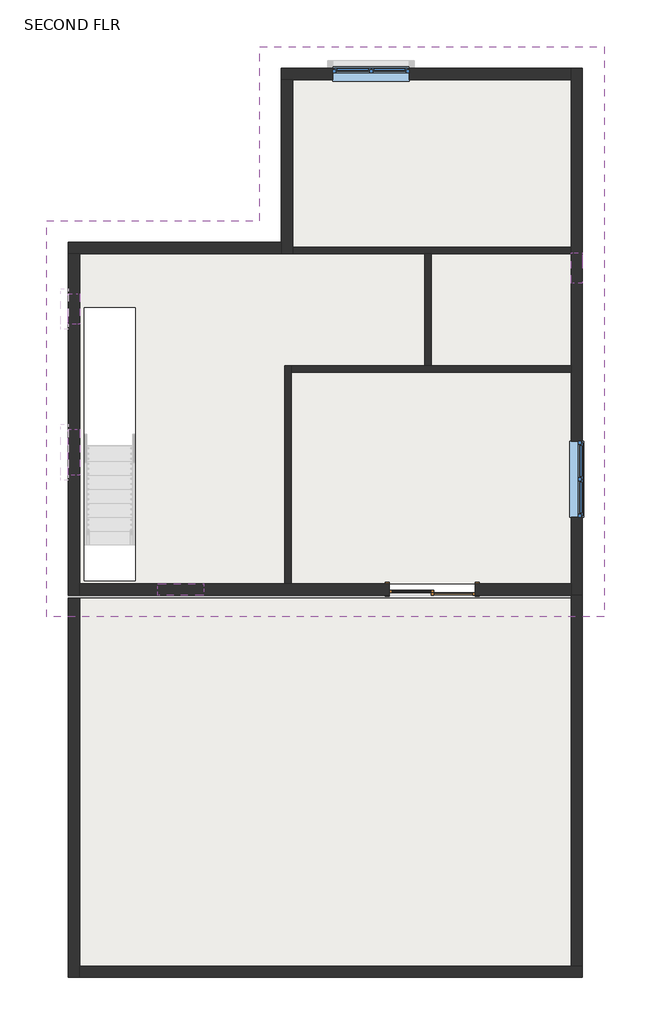
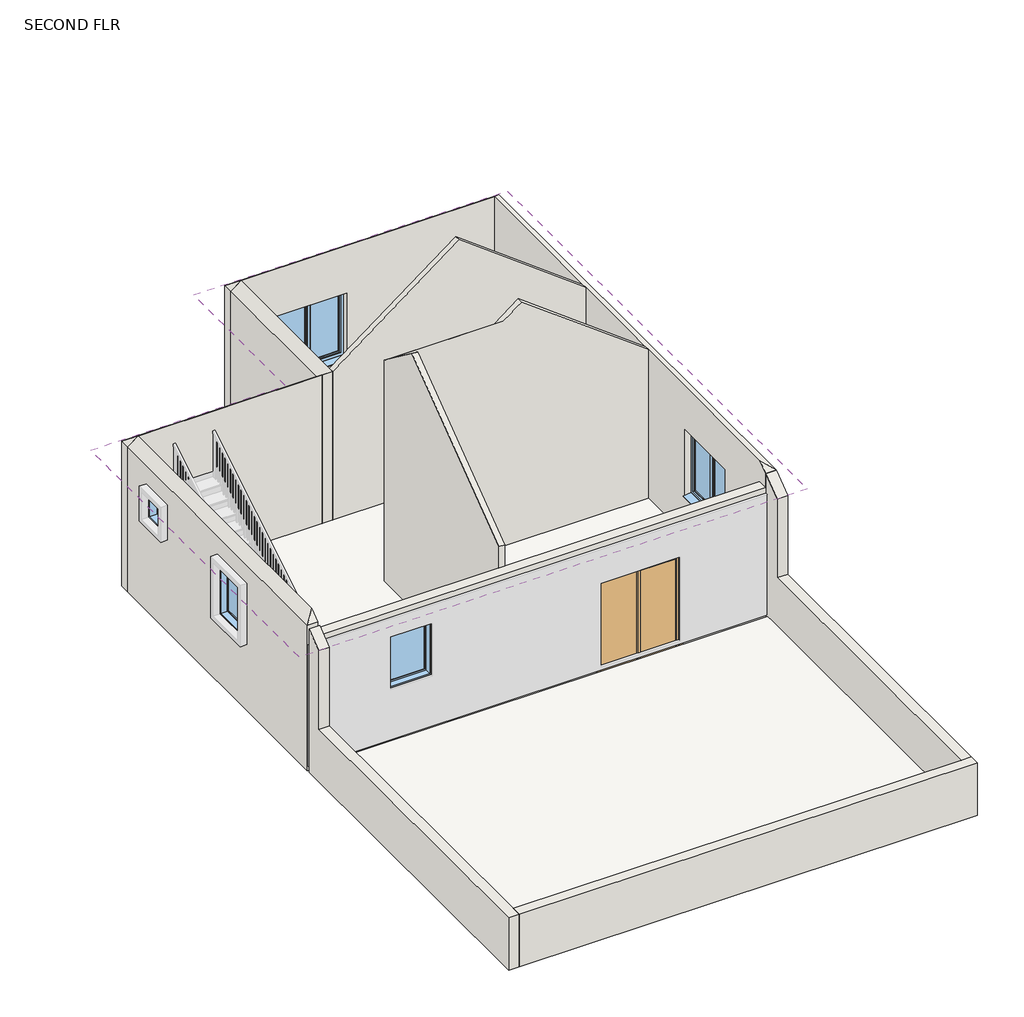
# One storey, part 1 of 2: 13 walls, 6 windows, 1 door, 1 roof, 1 slab.
"""IFC4 building model written with IfcOpenShell, lengths in millimetres."""

from ifc_helpers import new_model, si_unit, frame, origin, place, context, project, spatial, polyline, outline, extrude, faceted_brep, transform, mapped, element, save
from components import door_45189e27, window_80340324, fixed_window_3_x_3_dcb239d8, w2_windows_5_x_5_8ac21896

model = new_model("IFC4")

# Units and contexts
model_context = context("Model", 3, world=origin())
ifc_project = project(units=[si_unit("LENGTHUNIT", "METRE", prefix="MILLI")], contexts=[model_context])

# Site, building, storey
site = spatial("IfcSite", under=ifc_project)
building = spatial("IfcBuilding", under=site)
storey = spatial("IfcBuildingStorey", under=building, Name="SECOND FLR", Elevation=6400.8)

# Door
placement = place(None, origin())
door_shape = door_45189e27(model_context)
element("IfcDoor", 1, ObjectType="Door-Double-Sliding : 68\" x 84\"", at=placement, inside=storey, context=model_context, shape_type="MappedRepresentation", body=[
    mapped(door_shape, transform((1186.0219693, 1968.5641252, 6400.8), x_axis=(-1.0, 0.0, 0.0), y_axis=(0.0, -1.0, 0.0), z_axis=(0.0, 0.0, 1.0))),
])

# Roof
element("IfcRoof", 2, ObjectType="ROOFING 1'", at=placement, inside=storey, context=model_context, shape_type="Brep", body=[
    faceted_brep([(-2262.0280307, 9220.2641252, 9448.8), (-2262.0280307, 12700.0641252, 9448.8), (1179.6719693, 9258.3641252, 12030.075), (1179.6719693, 5778.5641252, 12030.075), (658.9719693, 5257.8641252, 12420.6), (-2566.8280307, 5257.8641252, 12420.6), (-6529.2280307, 9220.2641252, 9448.8), (4621.3719693, 12700.0641252, 9448.8), (-6529.2280307, 1295.4641252, 9448.8), (4621.3719693, 1295.4641252, 9448.8), (-2262.0280307, 9220.2641252, 9829.8), (1179.6719693, 5778.5641252, 12411.075), (1179.6719693, 9258.3641252, 12411.075), (-2262.0280307, 12700.0641252, 9829.8), (-6529.2280307, 9220.2641252, 9829.8), (-2566.8280307, 5257.8641252, 12801.6), (658.9719693, 5257.8641252, 12801.6), (4621.3719693, 12700.0641252, 9829.8), (-6529.2280307, 1295.4641252, 9829.8), (4621.3719693, 1295.4641252, 9829.8)], [[[0, 1, 2, 3]], [[0, 3, 4, 5, 6]], [[7, 2, 1]], [[8, 5, 4, 9]], [[6, 5, 8]], [[9, 4, 3, 2, 7]], [[10, 11, 12, 13]], [[10, 14, 15, 16, 11]], [[17, 13, 12]], [[18, 19, 16, 15]], [[14, 18, 15]], [[19, 17, 12, 11, 16]], [[6, 14, 10, 0]], [[8, 18, 14, 6]], [[9, 19, 18, 8]], [[7, 17, 19, 9]], [[1, 13, 17, 7]], [[0, 10, 13, 1]]]),
])

# Slab
element("IfcSlab", 3, ObjectType="MARBLE 6\"", at=placement, inside=storey, context=model_context, shape_type="SweptSolid", body=[
    extrude(outline(polyline([(3960.9719693, 12039.6641252), (3960.9719693, 8686.8641252), (-1601.6280307, 8686.8641252), (-1601.6280307, 12039.6641252), (3960.9719693, 12039.6641252)])), frame((0.0, 0.0, 6350.0), z_axis=(0.0, 0.0, 1.0), x_axis=(1.0, 0.0, 0.0)), (0.0, 0.0, 1.0), 152.4),
    extrude(outline(polyline([(3960.9719693, 8559.8641252), (3960.9719693, 6311.9641252), (1166.9719693, 6311.9641252), (1166.9719693, 8559.8641252), (3960.9719693, 8559.8641252)])), frame((0.0, 0.0, 6350.0), z_axis=(0.0, 0.0, 1.0), x_axis=(1.0, 0.0, 0.0)), (0.0, 0.0, 1.0), 152.4),
    extrude(outline(polyline([(3960.9719693, 1955.8641252), (-1639.7280307, 1955.8641252), (-1639.7280307, 6184.9641252), (3960.9719693, 6184.9641252), (3960.9719693, 1955.8641252)])), frame((0.0, 0.0, 6350.0), z_axis=(0.0, 0.0, 1.0), x_axis=(1.0, 0.0, 0.0)), (0.0, 0.0, 1.0), 152.4),
    extrude(outline(polyline([(1039.9719693, 8559.8641252), (1039.9719693, 6311.9641252), (-1766.7280307, 6311.9641252), (-1766.7280307, 1955.8641252), (-5868.7932997, 1955.8641252), (-5868.7932997, 8559.8641252), (1039.9719693, 8559.8641252)]), holes=[polyline([(-4756.3875748, 7481.7325341), (-5772.3875748, 7481.7325341), (-5772.3875748, 2020.7325341), (-4756.3875748, 2020.7325341), (-4756.3875748, 7481.7325341)])]), frame((0.0, 0.0, 6350.0), z_axis=(0.0, 0.0, 1.0), x_axis=(1.0, 0.0, 0.0)), (0.0, 0.0, 1.0), 152.4),
    extrude(outline(polyline([(-5868.7932997, 1663.7641252), (3960.9719693, 1663.7641252), (3960.9719693, -5689.5358748), (-5868.7932997, -5689.5358748), (-5868.7932997, 1663.7641252)])), frame((0.0, 0.0, 6350.0), z_axis=(0.0, 0.0, 1.0), x_axis=(1.0, 0.0, 0.0)), (0.0, 0.0, 1.0), 152.4),
])

# Walls
element("IfcWall", 4, ObjectType="INNER WALL5\"", at=placement, inside=storey, context=model_context, shape_type="Brep", body=[
    faceted_brep([(-1601.6280307, 8559.8641252, 6400.8), (1039.9719693, 8559.8641252, 6400.8), (1166.9719693, 8559.8641252, 6400.8), (3960.9719693, 8559.8641252, 6400.8), (3960.9719693, 8559.8641252, 9944.1), (1179.6719693, 8559.8641252, 12030.075), (-1601.6280307, 8559.8641252, 9944.1), (-1601.6280307, 8686.8641252, 6400.8), (-1601.6280307, 8686.8641252, 9944.1), (1179.6719693, 8686.8641252, 12030.075), (3960.9719693, 8686.8641252, 9944.1), (3960.9719693, 8686.8641252, 6400.8)], [[[0, 1, 2, 3, 4, 5, 6]], [[7, 8, 9, 10, 11]], [[3, 2, 1, 0, 7, 11]], [[4, 3, 11, 10]], [[0, 6, 8, 7]], [[6, 5, 9, 8]], [[5, 4, 10, 9]]]),
])
element("IfcWall", 5, ObjectType="INNER WALL5\"", at=placement, inside=storey, context=model_context, shape_type="Brep", body=[
    faceted_brep([(-1766.7280307, 6311.9641252, 6400.8), (-1766.7280307, 1955.8641252, 6400.8), (-1766.7280307, 1955.8641252, 9944.1), (-1766.7280307, 5257.8641252, 12420.6), (-1766.7280307, 6311.9641252, 11630.025), (-1639.7280307, 6311.9641252, 6400.8), (-1639.7280307, 6311.9641252, 11630.025), (-1639.7280307, 6184.9641252, 11725.275), (-1639.7280307, 5257.8641252, 12420.6), (-1639.7280307, 1955.8641252, 9944.1), (-1639.7280307, 1955.8641252, 6400.8), (-1639.7280307, 6184.9641252, 6400.8)], [[[0, 1, 2, 3, 4]], [[5, 6, 7, 8, 9, 10, 11]], [[1, 0, 5, 11, 10]], [[2, 1, 10, 9]], [[4, 3, 8, 7, 6]], [[3, 2, 9, 8]], [[0, 4, 6, 5]]]),
])
element("IfcWall", 6, ObjectType="INNER WALL5\"", at=placement, inside=storey, context=model_context, shape_type="Brep", body=[
    faceted_brep([(-1639.7280307, 6184.9641252, 6400.8), (3960.9719693, 6184.9641252, 6400.8), (3960.9719693, 6184.9641252, 9944.1), (1179.6719693, 6184.9641252, 12030.075), (773.2719693, 6184.9641252, 11725.275), (-1639.7280307, 6184.9641252, 11725.275), (-1639.7280307, 6311.9641252, 6400.8), (-1639.7280307, 6311.9641252, 11630.025), (646.2719693, 6311.9641252, 11630.025), (1179.6719693, 6311.9641252, 12030.075), (3960.9719693, 6311.9641252, 9944.1), (3960.9719693, 6311.9641252, 6400.8), (1166.9719693, 6311.9641252, 6400.8), (1039.9719693, 6311.9641252, 6400.8)], [[[0, 1, 2, 3, 4, 5]], [[6, 7, 8, 9, 10, 11, 12, 13]], [[1, 0, 6, 13, 12, 11]], [[2, 1, 11, 10]], [[5, 4, 8, 7]], [[4, 3, 9, 8]], [[3, 2, 10, 9]], [[0, 5, 7, 6]]]),
])
element("IfcWall", 7, ObjectType="INNER WALL5\"", at=placement, inside=storey, context=model_context, shape_type="SweptSolid", body=[
    extrude(outline(polyline([(1039.9719693, 6311.9641252), (1039.9719693, 8559.8641252), (1166.9719693, 8559.8641252), (1166.9719693, 6311.9641252), (1039.9719693, 6311.9641252)])), frame((0.0, 0.0, 6400.8), z_axis=(0.0, 0.0, 1.0), x_axis=(1.0, 0.0, 0.0)), (0.0, 0.0, 1.0), 3048.0),
])
element("IfcWall", 8, ObjectType="OUTER WALL 9\"", at=placement, inside=storey, context=model_context, shape_type="Brep", body=[
    faceted_brep([(4189.5719693, 1727.2641252, 9772.65), (4189.5719693, 1727.2641252, 6400.8), (4189.5719693, 12268.2641252, 6400.8), (4189.5719693, 12268.2641252, 9772.65), (4189.5719693, 3283.0141252, 7400.8), (4189.5719693, 3283.0141252, 8924.8), (4189.5719693, 4807.0141252, 8924.8), (4189.5719693, 4807.0141252, 7400.8), (4189.5719693, 8572.5641252, 8956.2819261), (4189.5719693, 8572.5641252, 8346.6819261), (4189.5719693, 7962.9641252, 8346.6819261), (4189.5719693, 7962.9641252, 8956.2819261), (3960.9719693, 1727.2641252, 6400.8), (3960.9719693, 1727.2641252, 9448.8), (3960.9719693, 1727.2641252, 9772.65), (3960.9719693, 1955.8641252, 9944.1), (3960.9719693, 6184.9641252, 9944.1), (3960.9719693, 6311.9641252, 9944.1), (3960.9719693, 8559.8641252, 9944.1), (3960.9719693, 8686.8641252, 9944.1), (3960.9719693, 12039.6641252, 9944.1), (3960.9719693, 12268.2641252, 9772.65), (3960.9719693, 12268.2641252, 6400.8), (3960.9719693, 12039.6641252, 6400.8), (3960.9719693, 8686.8641252, 6400.8), (3960.9719693, 8559.8641252, 6400.8), (3960.9719693, 6311.9641252, 6400.8), (3960.9719693, 6184.9641252, 6400.8), (3960.9719693, 1955.8641252, 6400.8), (3960.9719693, 3283.0141252, 7400.8), (3960.9719693, 4807.0141252, 7400.8), (3960.9719693, 4807.0141252, 8924.8), (3960.9719693, 3283.0141252, 8924.8), (3960.9719693, 8572.5641252, 8956.2819261), (3960.9719693, 7962.9641252, 8956.2819261), (3960.9719693, 7962.9641252, 8346.6819261), (3960.9719693, 8572.5641252, 8346.6819261)], [[[0, 1, 2, 3], [4, 5, 6, 7], [8, 9, 10, 11]], [[12, 13, 14, 15, 16, 17, 18, 19, 20, 21, 22, 23, 24, 25, 26, 27, 28], [29, 30, 31, 32], [33, 34, 35, 36]], [[2, 1, 12, 28, 27, 26, 25, 24, 23, 22]], [[3, 2, 22, 21]], [[0, 14, 13, 12, 1]], [[0, 3, 20, 19, 18, 17, 16, 15]], [[3, 21, 20]], [[15, 14, 0]], [[5, 4, 29, 32]], [[6, 5, 32, 31]], [[7, 6, 31, 30]], [[4, 7, 30, 29]], [[9, 8, 33, 36]], [[10, 9, 36, 35]], [[11, 10, 35, 34]], [[8, 11, 34, 33]]]),
])
element("IfcWall", 9, ObjectType="OUTER WALL 9\"", at=placement, inside=storey, context=model_context, shape_type="Brep", body=[
    faceted_brep([(3960.9719693, 12268.2641252, 6400.8), (-1830.2280307, 12268.2641252, 6400.8), (-1830.2280307, 12268.2641252, 9772.65), (3960.9719693, 12268.2641252, 9772.65), (722.4719693, 12268.2641252, 7315.2), (722.4719693, 12268.2641252, 8839.2), (-801.5280307, 12268.2641252, 8839.2), (-801.5280307, 12268.2641252, 7315.2), (3960.9719693, 12039.6641252, 6400.8), (3960.9719693, 12039.6641252, 9944.1), (-1601.6280307, 12039.6641252, 9944.1), (-1830.2280307, 12039.6641252, 9772.65), (-1830.2280307, 12039.6641252, 6400.8), (-1601.6280307, 12039.6641252, 6400.8), (722.4719693, 12039.6641252, 7315.2), (-801.5280307, 12039.6641252, 7315.2), (-801.5280307, 12039.6641252, 8839.2), (722.4719693, 12039.6641252, 8839.2)], [[[0, 1, 2, 3], [4, 5, 6, 7]], [[8, 9, 10, 11, 12, 13], [14, 15, 16, 17]], [[1, 0, 8, 13, 12]], [[0, 3, 9, 8]], [[2, 1, 12, 11]], [[3, 2, 10, 9]], [[2, 11, 10]], [[5, 4, 14, 17]], [[6, 5, 17, 16]], [[7, 6, 16, 15]], [[4, 7, 15, 14]]]),
])
element("IfcWall", 10, ObjectType="OUTER WALL 9\"", at=placement, inside=storey, context=model_context, shape_type="Brep", body=[
    faceted_brep([(-1830.2280307, 12039.6641252, 6400.8), (-1830.2280307, 8788.4641252, 6400.8), (-1830.2280307, 8559.8641252, 6400.8), (-1830.2280307, 8559.8641252, 9944.1), (-1830.2280307, 8788.4641252, 9772.65), (-1830.2280307, 12039.6641252, 9772.65), (-1601.6280307, 12039.6641252, 6400.8), (-1601.6280307, 12039.6641252, 9944.1), (-1601.6280307, 8686.8641252, 9944.1), (-1601.6280307, 8559.8641252, 9944.1), (-1601.6280307, 8559.8641252, 6400.8), (-1601.6280307, 8686.8641252, 6400.8)], [[[0, 1, 2, 3, 4, 5]], [[6, 7, 8, 9, 10, 11]], [[2, 1, 0, 6, 11, 10]], [[0, 5, 7, 6]], [[3, 2, 10, 9]], [[5, 4, 9, 8, 7]], [[4, 3, 9]]]),
])
element("IfcWall", 11, ObjectType="OUTER WALL 9\"", at=placement, inside=storey, context=model_context, shape_type="Brep", body=[
    faceted_brep([(-1830.2280307, 8788.4641252, 6400.8), (-6097.4280307, 8788.4641252, 6400.8), (-6097.4280307, 8788.4641252, 9772.65), (-1830.2280307, 8788.4641252, 9772.65), (-1830.2280307, 8559.8641252, 6400.8), (-1830.2280307, 8559.8641252, 9944.1), (-5868.8280307, 8559.8641252, 9944.1), (-6097.4280307, 8559.8641252, 9772.65), (-6097.4280307, 8559.8641252, 6400.8), (-5868.8280307, 8559.8641252, 6400.8)], [[[0, 1, 2, 3]], [[4, 5, 6, 7, 8, 9]], [[1, 0, 4, 9, 8]], [[0, 3, 5, 4]], [[2, 1, 8, 7]], [[3, 2, 6, 5]], [[2, 7, 6]]]),
])
element("IfcWall", 12, ObjectType="OUTER WALL 9\"", at=placement, inside=storey, context=model_context, shape_type="Brep", body=[
    faceted_brep([(-6097.4280307, 8559.8641252, 6400.8), (-6097.4280307, 1727.2641252, 6400.8), (-6097.4280307, 1727.2641252, 9772.65), (-6097.4280307, 8559.8641252, 9772.65), (-6097.4280307, 7150.1641252, 9237.9849297), (-6097.4280307, 7150.1641252, 8628.3849297), (-6097.4280307, 7759.7641252, 8628.3849297), (-6097.4280307, 7759.7641252, 9237.9849297), (-6097.4280307, 4127.5641252, 9252.2433359), (-6097.4280307, 4127.5641252, 8033.0433359), (-6097.4280307, 5041.9641252, 8033.0433359), (-6097.4280307, 5041.9641252, 9252.2433359), (-5868.8280307, 1727.2641252, 6400.8), (-5868.8280307, 1955.8641252, 6400.8), (-5868.8280307, 8559.8641252, 6400.8), (-5868.8280307, 8559.8641252, 9944.1), (-5868.8280307, 1955.8641252, 9944.1), (-5868.8280307, 1727.2641252, 9772.65), (-5868.8280307, 1727.2641252, 9448.8), (-5868.8280307, 7150.1641252, 8628.3849297), (-5868.8280307, 7150.1641252, 9237.9849297), (-5868.8280307, 7759.7641252, 9237.9849297), (-5868.8280307, 7759.7641252, 8628.3849297), (-5868.8280307, 4127.5641252, 9252.2433359), (-5868.8280307, 5041.9641252, 9252.2433359), (-5868.8280307, 5041.9641252, 8033.0433359), (-5868.8280307, 4127.5641252, 8033.0433359)], [[[0, 1, 2, 3], [4, 5, 6, 7], [8, 9, 10, 11]], [[12, 13, 14, 15, 16, 17, 18], [19, 20, 21, 22], [23, 24, 25, 26]], [[1, 0, 14, 13, 12]], [[0, 3, 15, 14]], [[2, 1, 12, 18, 17]], [[15, 3, 2, 16]], [[2, 17, 16]], [[5, 4, 20, 19]], [[6, 5, 19, 22]], [[7, 6, 22, 21]], [[4, 7, 21, 20]], [[9, 8, 23, 26]], [[10, 9, 26, 25]], [[11, 10, 25, 24]], [[8, 11, 24, 23]]]),
])
element("IfcWall", 13, ObjectType="OUTER WALL 9\"", at=placement, inside=storey, context=model_context, shape_type="Brep", body=[
    faceted_brep([(-5868.8280307, 1727.2641252, 6400.8), (322.4219693, 1727.2641252, 6400.8), (322.4219693, 1727.2641252, 8534.4), (2049.6219693, 1727.2641252, 8534.4), (2049.6219693, 1727.2641252, 6400.8), (3960.9719693, 1727.2641252, 6400.8), (3960.9719693, 1727.2641252, 9448.8), (-5868.8280307, 1727.2641252, 9448.8), (-3385.9780307, 1727.2641252, 8904.9782243), (-3385.9780307, 1727.2641252, 7685.7782243), (-4300.3780307, 1727.2641252, 7685.7782243), (-4300.3780307, 1727.2641252, 8904.9782243), (322.4219693, 1955.8641252, 8534.4), (322.4219693, 1955.8641252, 6400.8), (-1639.7280307, 1955.8641252, 6400.8), (-1766.7280307, 1955.8641252, 6400.8), (-5868.8280307, 1955.8641252, 6400.8), (-5868.8280307, 1955.8641252, 9448.8), (3960.9719693, 1955.8641252, 9448.8), (3960.9719693, 1955.8641252, 6400.8), (2049.6219693, 1955.8641252, 6400.8), (2049.6219693, 1955.8641252, 8534.4), (-3385.9780307, 1955.8641252, 8904.9782243), (-4300.3780307, 1955.8641252, 8904.9782243), (-4300.3780307, 1955.8641252, 7685.7782243), (-3385.9780307, 1955.8641252, 7685.7782243)], [[[0, 1, 2, 3, 4, 5, 6, 7], [8, 9, 10, 11]], [[12, 13, 14, 15, 16, 17, 18, 19, 20, 21], [22, 23, 24, 25]], [[20, 19, 5, 4]], [[16, 15, 14, 13, 1, 0]], [[7, 6, 18, 17]], [[6, 5, 19, 18]], [[0, 7, 17, 16]], [[4, 3, 21, 20]], [[2, 1, 13, 12]], [[3, 2, 12, 21]], [[9, 8, 22, 25]], [[10, 9, 25, 24]], [[11, 10, 24, 23]], [[8, 11, 23, 22]]]),
])
element("IfcWall", 14, ObjectType="OUTER WALL 9\"", at=placement, inside=storey, context=model_context, shape_type="Brep", body=[
    faceted_brep([(-6097.4280307, 1663.7641252, 6400.8), (-6097.4280307, -5918.1358748, 6400.8), (-6097.4280307, -5918.1358748, 7620.0), (-6097.4280307, 1295.4641252, 7620.0), (-6097.4280307, 1295.4641252, 9448.8), (-6097.4280307, 1663.7641252, 9725.025), (-5868.8280307, 1663.7641252, 6400.8), (-5868.8280307, 1663.7641252, 9725.025), (-5868.8280307, 1295.4641252, 9448.8), (-5868.8280307, 1295.4641252, 7620.0), (-5868.8280307, -5689.5358748, 7620.0), (-5868.8280307, -5918.1358748, 7620.0), (-5868.8280307, -5918.1358748, 6400.8), (-5868.8280307, -5689.5358748, 6400.8)], [[[0, 1, 2, 3, 4, 5]], [[6, 7, 8, 9, 10, 11, 12, 13]], [[1, 0, 6, 13, 12]], [[0, 5, 7, 6]], [[2, 1, 12, 11]], [[3, 2, 11, 10, 9]], [[3, 9, 8, 4]], [[5, 4, 8, 7]]]),
])
element("IfcWall", 15, ObjectType="OUTER WALL 9\"", at=placement, inside=storey, context=model_context, shape_type="Brep", body=[
    faceted_brep([(-5868.8280307, -5918.1358748, 6400.8), (4189.5719693, -5918.1358748, 6400.8), (4189.5719693, -5918.1358748, 7620.0), (-5868.8280307, -5918.1358748, 7620.0), (-5868.8280307, -5689.5358748, 6400.8), (-5868.8280307, -5689.5358748, 7620.0), (3960.9719693, -5689.5358748, 7620.0), (4189.5719693, -5689.5358748, 7620.0), (4189.5719693, -5689.5358748, 6400.8), (3960.9719693, -5689.5358748, 6400.8)], [[[0, 1, 2, 3]], [[4, 5, 6, 7, 8, 9]], [[1, 0, 4, 9, 8]], [[3, 2, 7, 6, 5]], [[0, 3, 5, 4]], [[2, 1, 8, 7]]]),
])
element("IfcWall", 16, ObjectType="OUTER WALL 9\"", at=placement, inside=storey, context=model_context, shape_type="SweptSolid", body=[
    extrude(outline(polyline([(-5689.5358748, 6400.8), (-5689.5358748, 7620.0), (1295.4641252, 7620.0), (1295.4641252, 9448.8), (1727.2641252, 9772.65), (1727.2641252, 6400.8), (-5689.5358748, 6400.8)])), frame((3960.9719693, 0.0, 0.0), z_axis=(1.0, 0.0, 0.0), x_axis=(0.0, 1.0, 0.0)), (0.0, 0.0, 1.0), 228.6),
])

# Windows
window_shape = window_80340324(model_context)
element("IfcWindow", 17, ObjectType="Fixed : 24\" x 24\"", at=placement, inside=storey, context=model_context, shape_type="MappedRepresentation", body=[
    mapped(window_shape, transform((4075.2719693, 8305.8641252, 7432.2819261), x_axis=(0.0, 1.0, 0.0), y_axis=(-1.0, 0.0, 0.0), z_axis=(0.0, 0.0, 1.0))),
])
element("IfcWindow", 18, ObjectType="Fixed : 24\" x 24\"", at=placement, inside=storey, context=model_context, shape_type="MappedRepresentation", body=[
    mapped(window_shape, transform((-5983.1280307, 7416.8641252, 7713.9849297), x_axis=(0.0, -1.0, 0.0), y_axis=(1.0, 0.0, 0.0), z_axis=(0.0, 0.0, 1.0))),
])
fixed_window_3_x_3_shape = fixed_window_3_x_3_dcb239d8(model_context)
element("IfcWindow", 19, ObjectType="Fixed : window 3' x 3'", at=placement, inside=storey, context=model_context, shape_type="MappedRepresentation", body=[
    mapped(fixed_window_3_x_3_shape, transform((-3805.0780307, 1841.5641252, 6771.3782243), x_axis=(1.0, 0.0, 0.0), y_axis=(0.0, 1.0, 0.0), z_axis=(0.0, 0.0, 1.0))),
])
element("IfcWindow", 20, ObjectType="Fixed : window 3' x 3'", at=placement, inside=storey, context=model_context, shape_type="MappedRepresentation", body=[
    mapped(fixed_window_3_x_3_shape, transform((-5983.1280307, 4546.6641252, 7118.6433359), x_axis=(0.0, -1.0, 0.0), y_axis=(1.0, 0.0, 0.0), z_axis=(0.0, 0.0, 1.0))),
])
w2_windows_5_x_5_shape = w2_windows_5_x_5_8ac21896(model_context)
element("IfcWindow", 21, ObjectType="w2 : WINDOWS 5' X 5'", at=placement, inside=storey, context=model_context, shape_type="MappedRepresentation", body=[
    mapped(w2_windows_5_x_5_shape, transform((4075.2719693, 4045.0141252, 6400.8), x_axis=(0.0, 1.0, 0.0), y_axis=(-1.0, 0.0, 0.0), z_axis=(0.0, 0.0, 1.0))),
])
element("IfcWindow", 22, ObjectType="w2 : WINDOWS 5' X 5'", at=placement, inside=storey, context=model_context, shape_type="MappedRepresentation", body=[
    mapped(w2_windows_5_x_5_shape, transform((-39.5280307, 12153.9641252, 6315.2), x_axis=(-1.0, 0.0, 0.0), y_axis=(0.0, -1.0, 0.0), z_axis=(0.0, 0.0, 1.0))),
])

save(model, "model.ifc")

# Revit data of these elements
# Type "Door-Double-Sliding : 68\" x 84\""
#   Type Mark = "9"
#   Construction Type Id = "opn-d45"
#   Assembly Code = "C1020"
#   Analytic Construction = "Wood frame, double glass door "
#   Thickness = 0' - 2"
#   Thermal Resistance (R) = 1.8150 (h·ft²·°F)/BTU
#   Heat Transfer Coefficient (U) = 0.5510 BTU/(h·ft²·°F)
#   Height = 7' - 0"
#   Rail Width = 0' - 2"
#   Stiles = 0' - 2"
#   Trim Projection Ext = 0' - 1"
#   Trim Projection Int = 0' - 1"
#   Trim Width = 0' - 3"
#   Width = 5' - 8"
#   Define Thermal Properties by = 1
#   Glazing = Glass
#   Panel Material = Wood - Birch - Solid Stained Light Low Gloss
#   Trim Material = Paint - Sienna
#   Visual Light Transmittance = 0
#   Solar Heat Gain Coefficient = 0
#   Function = (empty or 0)
#   Wall Closure = (empty or 0)
# Type "ROOFING 1'"
#   Assembly Code = "B1020"
#   Layers, outside or top first: 1' - 0" "ROOFING PAINT" (function 1)
# Type "MARBLE 6\""
#   Assembly Code = "B1010"
#   Function = 0
#   Layers, outside or top first: 0' - 6" "MARBLE MATERIAL" (function 1)
# Type "INNER WALL5\""
#   Assembly Code = "B2010"
#   Layers, outside or top first: 0' - 5" "OUTER WALL 9\"" (function 1)
# Type "OUTER WALL 9\""
#   Assembly Code = "B2010"
#   Layers, outside or top first: 0' - 9" "OUTER WALL 9\"" (function 1)
# Type "Fixed : 24\" x 24\""
#   Type Mark = "3"
#   Construction Type Id = "GSP4R"
#   Assembly Code = "B2020100"
#   Analytic Construction = "1/8 in Pilkington single glazing"
#   Visual Light Transmittance = 0.9
#   Solar Heat Gain Coefficient = 0.78
#   Heat Transfer Coefficient (U) = 0.6496 BTU/(h·ft²·°F)
#   Height = 2' - 0"
#   Default Sill Height = 3' - 0"
#   Width = 2' - 0"
#   Window Inset = 0' - 0 3/4"
#   Define Thermal Properties by = 1
#   Define Thermal Properties by = 1
#   Glass Pane Material = Glass
#   Sash Material = Sash
#   Wall Closure = (empty or 0)
# Type "Fixed : window 3' x 3'"
#   Type Mark = "18"
#   Construction Type Id = "GSP4R"
#   Assembly Code = "B2020100"
#   Analytic Construction = "1/8 in Pilkington single glazing"
#   Visual Light Transmittance = 0.9
#   Solar Heat Gain Coefficient = 0.78
#   Heat Transfer Coefficient (U) = 0.6496 BTU/(h·ft²·°F)
#   Height = 4' - 0"
#   Default Sill Height = 3' - 0"
#   Width = 3' - 0"
#   Window Inset = 0' - 2"
#   Define Thermal Properties by = 1
#   Glass Pane Material = Glass
#   Sash Material = Sash
#   Wall Closure = (empty or 0)
# Type "w2 : WINDOWS 5' X 5'"
#   Type Mark = "26"
#   Operation = "DoublePanelVertical"
#   Keynote = "16.05.01"
#   Analytic Construction = "<None>"
#   Rough Width = 5' - 0"
#   Rough Height = 5' - 0"
#   Rahmentiefe = 0' - 2.3622"
#   Rahmenhöhe unten = 0' - 3.14961"
#   Rahmehöhe oben = 0' - 3.14961"
#   Rahmenbreite = 0' - 2.3622"
#   Heat Transfer Coefficient (U) = 2.81836 BTU/(h·ft²·°F)
#   Height = 5' - 0"
#   Flügeltiefe = 0' - 2.3622"
#   Flügelbreite = 0' - 2.3622"
#   Einbautiefe (von außen) [instance default] = 0' - 5.51181"
#   Width = 5' - 0"
#   Kippflügel [instance default] = yes
#   Drehflügel im Grundriß darstellen [instance default] = no
#   Drehflügel [instance default] = yes
#   Define Thermal Properties by = 1
#   Rahmen [instance default] = none
#   Glas [instance default] = blue glass
#   Flügel [instance default] = WINDOW COLOUR WHITE
#   Fensterbank aussen [instance default] = WINDOW COLOUR WHITE
#   Fensterbank innen [instance default] = WINDOW COLOUR WHITE
#   Visual Light Transmittance = 0
#   Thermal Resistance (R) = 0
#   Solar Heat Gain Coefficient = 0
#   Wall Closure = (empty or 0)
# Element 1 (IfcDoor, "Door-Double-Sliding : 68\" x 84\"")
#   Phase Created = New Construction
#   Materials on its faces: "Paint - Sienna", "Wood - Birch - Solid Stained Light Low Gloss", "Glass"
# Element 2 (IfcRoof, "ROOFING 1'")
#   built-in parameter 1001705 = 42 (stored number, unit not read)
#   built-in parameter 1001701 = 10 (stored number, unit not read)
#   built-in parameter 1001710 = 33615
#   Phase Created = New Construction
#   Materials on its faces: "ROOFING PAINT"
# Element 3 (IfcSlab, "MARBLE 6\"")
#   Height Offset From Level = 0' - 4"
#   Phase Created = New Construction
#   Materials on its faces: "MARBLE MATERIAL"
# Elements 4, 5, 6 (IfcWall, "INNER WALL5\"")
#   Top Offset = 0' - 0"
#   Base Offset = 0' - 0"
#   Unconnected Height = 10' - 0"
#   wall height = 10' - 0"
#   Phase Created = New Construction
#   Base Constraint = SECOND FLR
#   Materials on its faces: "OUTER WALL 9\""
# Element 7 (IfcWall, "INNER WALL5\"")
#   Top Offset = 0' - 0"
#   Base Offset = 0' - 0"
#   wall height = 10' - 0"
#   Phase Created = New Construction
#   Base Constraint = SECOND FLR
#   Top Constraint = TOP OF ROOF
#   Materials on its faces: "OUTER WALL 9\""
# Elements 8, 9, 10, 11, 12 (IfcWall, "OUTER WALL 9\"")
#   Top Offset = 0' - 0"
#   Base Offset = 0' - 0"
#   Unconnected Height = 10' - 0"
#   wall height = 10' - 0"
#   Phase Created = New Construction
#   Base Constraint = SECOND FLR
#   Materials on its faces: "OUTER WALL 9\""
# Element 13 (IfcWall, "OUTER WALL 9\"")
#   Top Offset = 0' - 0"
#   Base Offset = 0' - 0"
#   wall height = 10' - 0"
#   Phase Created = New Construction
#   Base Constraint = SECOND FLR
#   Top Constraint = TOP OF ROOF
#   Materials on its faces: "OUTER WALL 9\""
# Elements 14, 15, 16 (IfcWall, "OUTER WALL 9\"")
#   Top Offset = 0' - 0"
#   Base Offset = 0' - 0"
#   Unconnected Height = 4' - 0"
#   wall height = 4' - 0"
#   Phase Created = New Construction
#   Base Constraint = SECOND FLR
#   Materials on its faces: "OUTER WALL 9\""
# Element 17 (IfcWindow, "Fixed : 24\" x 24\"")
#   Mark = "6"
#   Phase Created = New Construction
#   Materials on its faces: "Sash", "Glass"
# Element 18 (IfcWindow, "Fixed : 24\" x 24\"")
#   Mark = "11"
#   Phase Created = New Construction
#   Materials on its faces: "Sash", "Glass"
# Element 19 (IfcWindow, "Fixed : window 3' x 3'")
#   Mark = "2"
#   Phase Created = New Construction
#   Materials on its faces: "Sash", "Glass"
# Element 20 (IfcWindow, "Fixed : window 3' x 3'")
#   Mark = "15"
#   Phase Created = New Construction
#   Materials on its faces: "Sash", "Glass"
# Element 21 (IfcWindow, "w2 : WINDOWS 5' X 5'")
#   Mark = "5"
#   Einbautiefe (von außen) = 0' - 5.51181"
#   Kippflügel = yes
#   Drehflügel im Grundriß darstellen = no
#   Drehflügel = yes
#   Rahmen = none
#   Glas = blue glass
#   Flügel = WINDOW COLOUR WHITE
#   Fensterbank innen = WINDOW COLOUR WHITE
#   Fensterbank aussen = WINDOW COLOUR WHITE
#   Phase Created = New Construction
#   Materials on its faces: "WINDOW COLOUR WHITE", "blue glass"
# Element 22 (IfcWindow, "w2 : WINDOWS 5' X 5'")
#   Mark = "10"
#   Einbautiefe (von außen) = 0' - 5.51181"
#   Kippflügel = yes
#   Drehflügel im Grundriß darstellen = no
#   Drehflügel = yes
#   Rahmen = none
#   Glas = blue glass
#   Flügel = WINDOW COLOUR WHITE
#   Fensterbank innen = WINDOW COLOUR WHITE
#   Fensterbank aussen = WINDOW COLOUR WHITE
#   Phase Created = New Construction
#   Materials on its faces: "WINDOW COLOUR WHITE", "blue glass"
# Materials
#   "Glass": class "Glass", colour RGB 0 128 192, transparency 0.75, Description = "Soda Lime Glass", Cost = 0
#   "Wood - Birch - Solid Stained Light Low Gloss": class "Wood", colour RGB 210 159 95, transparency 0, Cost = 0
#   "Paint - Sienna": colour RGB 118 70 51, transparency 0, Cost = 0
#   "ROOFING PAINT": class "Generic", colour RGB 120 120 120, transparency 0, Cost = 0
#   "MARBLE MATERIAL": class "Generic", colour RGB 120 120 120, transparency 0, Cost = 0
#   "OUTER WALL 9\"": class "Generic", colour RGB 120 120 120, transparency 0, Cost = 0
#   "Sash": class "Wood", colour RGB 224 178 126, transparency 0, Cost = 0
#   "blue glass": class "System", colour RGB 0 0 255, transparency 0.75, Cost = 0
#   "WINDOW COLOUR WHITE": class "Generic", colour RGB 120 120 120, transparency 0, Cost = 0
